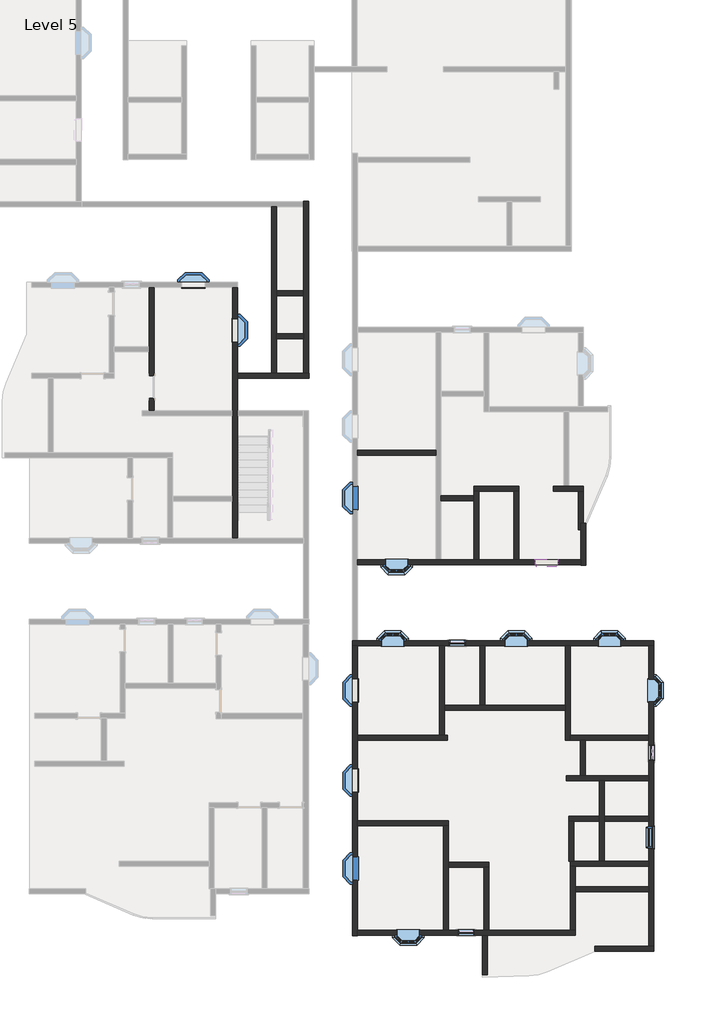
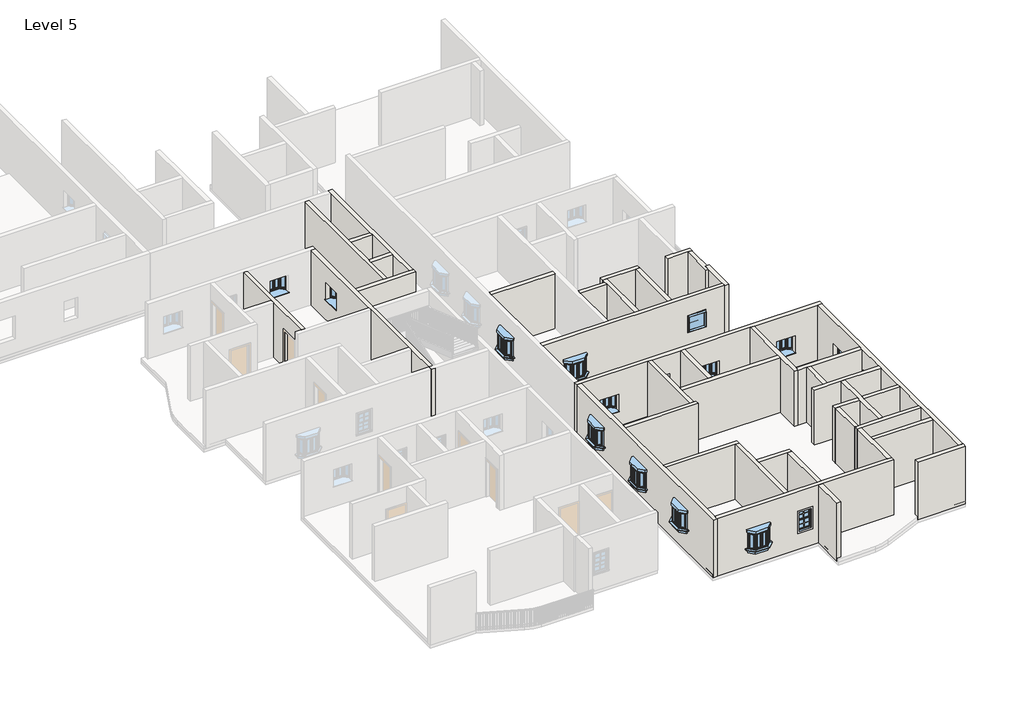
# One storey, part 2 of 14: 40 walls, 17 windows.
# Revit data of these elements (continued)
# Element 46 (IfcWindow, "910x910mm") (continued)
#   Materials on its faces: "Window Frame", "Glass"
# Element 47 (IfcWindow, "910x910mm")
#   Mark = "244"
#   Phase Created = New Construction
#   Materials on its faces: "Window Frame", "Glass"
# Element 48 (IfcWindow, "910x910mm")
#   Mark = "245"
#   Phase Created = New Construction
#   Materials on its faces: "Window Frame", "Glass"
# Element 49 (IfcWindow, "910x910mm")
#   Mark = "246"
#   Phase Created = New Construction
#   Materials on its faces: "Window Frame", "Glass"
# Element 50 (IfcWindow, "910x910mm")
#   Mark = "247"
#   Phase Created = New Construction
#   Materials on its faces: "Window Frame", "Glass"
# Element 51 (IfcWindow, "910x910mm")
#   Mark = "248"
#   Phase Created = New Construction
#   Materials on its faces: "Window Frame", "Glass"
# Element 52 (IfcWindow, "910x910mm")
#   Mark = "249"
#   Phase Created = New Construction
#   Materials on its faces: "Window Frame", "Glass"
# Element 53 (IfcWindow, "Window-Double-Hung : 26\" x 42\"")
#   Mark = "272"
#   Window Inset = 0' - 0"
#   Interior Wall Closure = 0' - 1 1/2"
#   Frame Extension = 0' - 1 1/4"
#   Exterior Wall Closure = 0' - 0 1/2"
#   Interior Trim Visibility = yes
#   Indicator Visibility = yes
#   Exterior Trim Visibility = yes
#   Phase Created = New Construction
#   Materials on its faces: "Wood - Stained", "Glass", "Clad - White"
# Element 54 (IfcWindow, "Window-Double-Hung : 26\" x 42\"")
#   Mark = "273"
#   Window Inset = 0' - 0"
#   Interior Wall Closure = 0' - 1 1/2"
#   Frame Extension = 0' - 1 1/4"
#   Exterior Wall Closure = 0' - 0 1/2"
#   Interior Trim Visibility = yes
#   Indicator Visibility = yes
#   Exterior Trim Visibility = yes
#   Phase Created = New Construction
#   Materials on its faces: "Wood - Stained", "Glass", "Clad - White"
# Element 55 (IfcWindow, "Window-Double-Hung : 26\" x 42\"")
#   Mark = "274"
#   Window Inset = 0' - 0"
#   Interior Wall Closure = 0' - 1 1/2"
#   Frame Extension = 0' - 1 1/4"
#   Exterior Wall Closure = 0' - 0 1/2"
#   Interior Trim Visibility = yes
#   Indicator Visibility = yes
#   Exterior Trim Visibility = yes
#   Phase Created = New Construction
#   Materials on its faces: "Wood - Stained", "Glass", "Clad - White"
# Element 56 (IfcWindow, "Windows_Sgl_w-Glazing_Bars : 910x910mm")
#   Mark = "262"
#   Phase Created = New Construction
#   Materials on its faces: "Window Frame", "Glass"
# Element 57 (IfcWindow, "Windows_Sgl_w-Glazing_Bars : 910x910mm")
#   Mark = "261"
#   Phase Created = New Construction
#   Materials on its faces: "Window Frame", "Glass"
# Materials
#   "Window Frame": colour RGB 249 249 249, transparency 0
#   "Glass": class "Glass", colour RGB 0 128 192, transparency 0.75, Description = "Soda Lime Glass", Cost = 0
#   "Wood - Stained": class "Wood", colour RGB 224 178 126, transparency 0, Cost = 0
#   "Clad - White": class "Wood", colour RGB 242 242 238, transparency 0, Cost = 0
#   "Default Wall": colour RGB 128 128 128, transparency 0, Cost = 0
#   "Door - Frame": colour RGB 118 70 51, transparency 0, Cost = 0
#   "Earth": class "Generic", colour RGB 97 75 62, transparency 0, Description = "Soil", Cost = 0
#   "Carpet (1)": class "Carpet", colour RGB 124 80 67, transparency 0, Description = "Interior finish", Cost = 0
#   "Acoustic Ceiling Tile 24 x 24": class "Generic", colour RGB 232 232 232, transparency 0, Description = "Acoustic Ceiling Tile 24 x 24", Cost = 0
